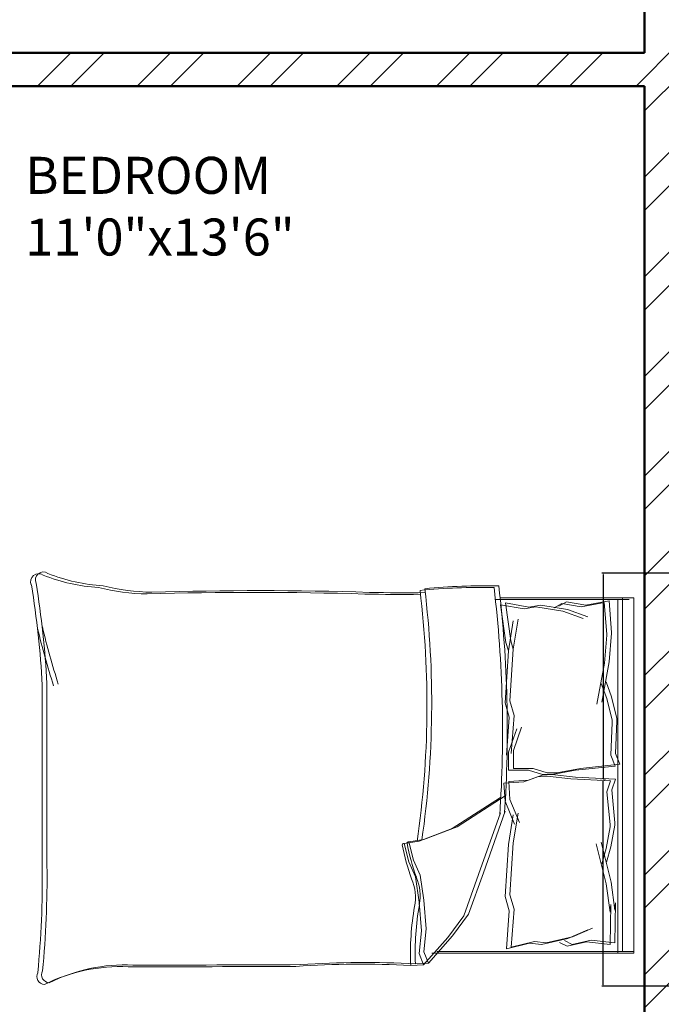
# Model space of a CAD drawing. Units: inches. Extents: x 963 to 2075, y 289 to 2657.
# Tile 12 of 98: x 1424 to 1511, y 1585 to 1718. Entities that reach past the tile are written whole.
import ezdxf

# ---------------------------------------------------------------- set-up
doc = ezdxf.new("R2010")
doc.units = ezdxf.units.IN
for name, color, linetype, lineweight in [('A-ANNO-DIMS', 2, 'Continuous', 18), ('A-AREA-IDEN', 7, 'Continuous', 18), ('A-FURN', 8, 'Continuous', 18), ('A-WALL', 7, 'Continuous', 50), ('A-WALL-PATT', 8, 'Continuous', 13)]:
    doc.layers.add(name, color=color, linetype=linetype, lineweight=lineweight)
doc.styles.get("Standard").update_dxf_attribs({"font": 'arial.ttf'})
doc.dimstyles.get("Standard").update_dxf_attribs({"dimtxt": 0.18, "dimasz": 0.18, "dimexe": 0.18, "dimexo": 0.0625, "dimgap": 0.09, "dimtad": 0, "dimtih": 1, "dimtoh": 1, "dimdec": 4, "dimzin": 0, "dimdsep": 46, "dimtxsty": 'Standard', "dimcen": 0.09, "dimadec": 0, "dimazin": 0, "dimtfac": 1, "dimtdec": 4, "dimtofl": 0, "dimtmove": 0, "dimatfit": 3, "dimfxl": 1, "dimtolj": 1, "dimtzin": 0, "dimarcsym": 0})

# ---------------------------------------------------------------- blocks, each defined once
blk = doc.blocks.new('BED-DOUBLE')
for p, q in [((1236.12, 2450.52), (1254.23, 2450.52)), ((1236.12, 2450.52), (1254.23, 2450.52)), ((1236.76, 2450.75), (1254.87, 2450.75)), ((1236.76, 2450.75), (1254.87, 2450.75)), ((1237.61, 2444.71), (1236.89, 2449.81)), ((1236.89, 2449.81), (1240.07, 2449.23)), ((1237.61, 2444.71), (1236.89, 2449.81)), ((1236.89, 2449.81), (1240.07, 2449.23)), ((1238.25, 2444.94), (1237.53, 2450.04)), ((1237.53, 2450.04), (1240.71, 2449.46)), ((1238.25, 2444.94), (1237.53, 2450.04)), ((1237.53, 2450.04), (1240.71, 2449.46)), ((1240.07, 2449.23), (1241.66, 2449.52)), ((1240.07, 2449.23), (1241.66, 2449.52)), ((1240.71, 2449.46), (1242.3, 2449.75)), ((1240.71, 2449.46), (1242.3, 2449.75)), ((1241.66, 2449.52), (1245.28, 2448.94)), ((1241.66, 2449.52), (1245.28, 2448.94)), ((1242.3, 2449.75), (1245.92, 2449.17)), ((1242.3, 2449.75), (1245.92, 2449.17)), ((1245.13, 2449.96), (1244.12, 2449.38)), ((1245.13, 2449.96), (1244.12, 2449.38)), ((1245.77, 2450.18), (1244.76, 2449.61)), ((1245.77, 2450.18), (1244.76, 2449.61)), ((1247.74, 2449.52), (1245.13, 2449.96)), ((1247.74, 2449.52), (1245.13, 2449.96)), ((1248.37, 2449.75), (1245.77, 2450.18)), ((1248.37, 2449.75), (1245.77, 2450.18)), ((1250.92, 2450.1), (1247.74, 2449.52)), ((1250.92, 2450.1), (1247.74, 2449.52)), ((1251.56, 2450.33), (1248.37, 2449.75)), ((1251.56, 2450.33), (1248.37, 2449.75)), ((1250.89, 2450.1), (1251.22, 2445.82)), ((1250.89, 2450.1), (1251.22, 2445.82)), ((1251.53, 2450.32), (1251.86, 2446.04)), ((1251.53, 2450.32), (1251.86, 2446.04)), ((1252.7, 2450.52), (1252.7, 2402.73)), ((1252.7, 2450.52), (1252.7, 2402.73)), ((1253.34, 2450.75), (1253.34, 2402.96)), ((1253.34, 2450.75), (1253.34, 2402.96)), ((1254.87, 2450.75), (1254.87, 2402.73)), ((1245.28, 2448.94), (1248.02, 2447.93)), ((1245.28, 2448.94), (1248.02, 2447.93)), ((1245.92, 2449.17), (1248.66, 2448.16)), ((1245.92, 2449.17), (1248.66, 2448.16)), ((1238.6, 2447.61), (1237.94, 2443.58)), ((1238.6, 2447.61), (1237.94, 2443.58)), ((1239.24, 2447.84), (1238.58, 2443.81)), ((1239.24, 2447.84), (1238.58, 2443.81)), ((1251.21, 2445.71), (1250.92, 2441.89)), ((1251.21, 2445.71), (1250.92, 2441.89)), ((1251.22, 2445.82), (1251.21, 2445.71)), ((1251.22, 2445.82), (1251.21, 2445.71)), ((1251.84, 2445.94), (1251.56, 2442.11)), ((1251.84, 2445.94), (1251.56, 2442.11)), ((1251.86, 2446.04), (1251.84, 2445.94)), ((1251.86, 2446.04), (1251.84, 2445.94)), ((1237.94, 2443.58), (1237.61, 2444.71)), ((1237.94, 2443.58), (1237.61, 2444.71)), ((1238.58, 2443.81), (1238.25, 2444.94)), ((1238.58, 2443.81), (1238.25, 2444.94)), ((1237.94, 2443.58), (1237.51, 2436.57)), ((1237.94, 2443.58), (1237.51, 2436.57)), ((1238.58, 2443.81), (1238.15, 2436.8)), ((1238.58, 2443.81), (1238.15, 2436.8)), ((1250.92, 2441.89), (1249.9, 2436.39)), ((1250.92, 2441.89), (1249.9, 2436.39)), ((1251.56, 2442.11), (1250.54, 2436.62)), ((1251.56, 2442.11), (1250.54, 2436.62)), ((1174.99, 2438.93), (1174.99, 2414.32)), ((1174.99, 2438.93), (1174.99, 2414.32)), ((1175.63, 2439.16), (1175.63, 2414.55)), ((1175.63, 2439.16), (1175.63, 2414.55)), ((1250.48, 2439.14), (1251.21, 2437.12)), ((1250.48, 2439.14), (1251.21, 2437.12)), ((1251.12, 2439.37), (1251.84, 2437.34)), ((1251.12, 2439.37), (1251.84, 2437.34)), ((1237.51, 2436.57), (1238.06, 2434.61)), ((1237.51, 2436.57), (1238.06, 2434.61)), ((1238.15, 2436.8), (1238.7, 2434.84)), ((1238.15, 2436.8), (1238.7, 2434.84)), ((1251.21, 2437.12), (1251.93, 2434.22)), ((1251.21, 2437.12), (1251.93, 2434.23)), ((1251.84, 2437.34), (1252.57, 2434.45)), ((1251.84, 2437.34), (1252.57, 2434.45)), ((1238.06, 2434.61), (1237.66, 2429.48)), ((1238.06, 2434.61), (1237.66, 2429.48)), ((1238.7, 2434.84), (1238.3, 2429.71)), ((1238.7, 2434.84), (1238.3, 2429.71)), ((1251.93, 2433.9), (1251.78, 2429.46)), ((1251.93, 2433.9), (1251.78, 2429.46)), ((1251.93, 2434.23), (1251.93, 2433.9)), ((1251.93, 2434.22), (1251.93, 2433.9)), ((1252.57, 2434.13), (1252.42, 2429.69)), ((1252.57, 2434.13), (1252.42, 2429.69)), ((1252.57, 2434.45), (1252.57, 2434.13)), ((1252.57, 2434.45), (1252.57, 2434.13)), ((1237.97, 2429.89), (1239.06, 2433.04)), ((1237.97, 2429.89), (1239.06, 2433.04)), ((1238.61, 2430.12), (1239.7, 2433.26)), ((1238.61, 2430.12), (1239.7, 2433.26)), ((1237.97, 2427.43), (1237.97, 2429.89)), ((1237.97, 2427.43), (1237.97, 2429.89)), ((1238.61, 2427.66), (1238.61, 2430.12)), ((1238.61, 2427.66), (1238.61, 2430.12)), ((1252.42, 2429.69), (1253, 2428.24)), ((1252.42, 2429.69), (1253, 2428.24)), ((1253, 2428.24), (1247.65, 2427.66)), ((1253, 2428.24), (1247.65, 2427.66)), ((1251.78, 2429.46), (1252.36, 2428.01)), ((1251.78, 2429.46), (1252.36, 2428.01)), ((1240.65, 2427.43), (1237.97, 2427.43)), ((1240.65, 2427.43), (1237.97, 2427.43)), ((1241.29, 2427.66), (1238.61, 2427.66)), ((1241.29, 2427.66), (1238.61, 2427.66)), ((1242.53, 2426.86), (1240.65, 2427.43)), ((1242.53, 2426.86), (1240.65, 2427.43)), ((1243.17, 2427.08), (1241.29, 2427.66)), ((1243.17, 2427.08), (1241.29, 2427.66)), ((1244.47, 2427.08), (1243.17, 2427.08)), ((1244.47, 2427.08), (1243.17, 2427.08)), ((1247.01, 2427.43), (1243.83, 2426.86)), ((1247.01, 2427.43), (1243.83, 2426.86)), ((1247.65, 2427.66), (1244.47, 2427.08)), ((1247.65, 2427.66), (1244.47, 2427.08)), ((1252.36, 2428.01), (1247.01, 2427.43)), ((1252.36, 2428.01), (1247.01, 2427.43)), ((1240.02, 2425.86), (1237.34, 2425.7)), ((1240.02, 2425.86), (1237.34, 2425.7)), ((1237.34, 2425.7), (1237.49, 2423.24)), ((1237.34, 2425.7), (1237.49, 2423.24)), ((1240.66, 2426.09), (1237.98, 2425.93)), ((1240.66, 2426.09), (1237.98, 2425.93)), ((1237.98, 2425.93), (1238.13, 2423.47)), ((1237.98, 2425.93), (1238.13, 2423.47)), ((1241.86, 2426.56), (1240.02, 2425.86)), ((1241.86, 2426.56), (1240.02, 2425.86)), ((1242.49, 2426.79), (1240.66, 2426.09)), ((1242.49, 2426.79), (1240.66, 2426.09)), ((1243.15, 2426.64), (1241.86, 2426.56)), ((1243.15, 2426.64), (1241.86, 2426.56)), ((1243.79, 2426.87), (1242.49, 2426.79)), ((1243.79, 2426.87), (1242.49, 2426.79)), ((1243.83, 2426.86), (1242.53, 2426.86)), ((1243.83, 2426.86), (1242.53, 2426.86)), ((1246.37, 2426.26), (1243.15, 2426.64)), ((1246.37, 2426.26), (1243.15, 2426.64)), ((1247, 2426.49), (1243.79, 2426.87)), ((1247, 2426.49), (1243.79, 2426.87)), ((1251.74, 2426.02), (1246.37, 2426.26)), ((1251.74, 2426.02), (1246.37, 2426.26)), ((1252.38, 2426.25), (1247, 2426.49)), ((1252.38, 2426.25), (1247, 2426.49)), ((1251.25, 2424.54), (1251.74, 2426.02)), ((1251.25, 2424.54), (1251.74, 2426.02)), ((1251.89, 2424.77), (1252.38, 2426.25)), ((1251.89, 2424.77), (1252.38, 2426.25)), ((1251.68, 2420.11), (1251.25, 2424.54)), ((1251.68, 2420.11), (1251.25, 2424.54)), ((1252.31, 2420.34), (1251.89, 2424.77)), ((1252.31, 2420.34), (1251.89, 2424.77)), ((1236.85, 2423.74), (1230.36, 2419.55)), ((1236.85, 2423.74), (1230.36, 2419.55)), ((1237.49, 2423.96), (1231, 2419.77)), ((1237.49, 2423.96), (1231, 2419.77)), ((1237.49, 2423.24), (1238.78, 2420.17)), ((1237.49, 2423.24), (1238.78, 2420.17)), ((1238.13, 2423.47), (1239.42, 2420.4)), ((1238.13, 2423.47), (1239.42, 2420.4)), ((1233.92, 2413.35), (1236.85, 2421.69)), ((1233.92, 2413.35), (1236.85, 2421.69)), ((1234.56, 2413.58), (1237.49, 2421.92)), ((1234.56, 2413.58), (1237.49, 2421.92)), ((1239.24, 2421.66), (1238.58, 2417.63)), ((1239.24, 2421.66), (1238.58, 2417.63)), ((1238.6, 2421.43), (1237.94, 2417.4)), ((1238.6, 2421.43), (1237.94, 2417.4)), ((1252.33, 2420.02), (1252.31, 2420.34)), ((1252.33, 2420.02), (1252.31, 2420.34)), ((1230.36, 2419.55), (1225.87, 2417.84)), ((1230.36, 2419.55), (1225.87, 2417.84)), ((1231, 2419.77), (1226.51, 2418.07)), ((1231, 2419.77), (1226.51, 2418.07)), ((1251.15, 2416.86), (1251.7, 2419.79)), ((1251.15, 2416.86), (1251.7, 2419.79)), ((1251.7, 2419.79), (1251.68, 2420.11)), ((1251.7, 2419.79), (1251.68, 2420.11)), ((1251.79, 2417.09), (1252.33, 2420.02)), ((1251.79, 2417.09), (1252.33, 2420.02)), ((1225.87, 2417.84), (1223.86, 2417.53)), ((1225.87, 2417.84), (1223.86, 2417.53)), ((1226.51, 2418.07), (1224.49, 2417.76)), ((1226.51, 2418.07), (1224.49, 2417.76)), ((1224.49, 2417.76), (1225.11, 2415.28)), ((1224.49, 2417.76), (1225.11, 2415.28)), ((1238.58, 2417.63), (1238.15, 2410.62)), ((1238.58, 2417.63), (1238.15, 2410.62)), ((1251.8, 2412.31), (1250.45, 2417.73)), ((1251.8, 2412.31), (1250.45, 2417.73)), ((1223.86, 2417.53), (1224.47, 2415.05)), ((1223.86, 2417.53), (1224.47, 2415.05)), ((1237.94, 2417.4), (1237.51, 2410.39)), ((1237.94, 2417.4), (1237.51, 2410.39)), ((1251.16, 2412.08), (1249.81, 2417.5)), ((1251.16, 2412.08), (1249.81, 2417.5)), ((1250.56, 2414.79), (1251.15, 2416.86)), ((1250.56, 2414.79), (1251.15, 2416.86)), ((1251.2, 2415.02), (1251.79, 2417.09)), ((1251.2, 2415.02), (1251.79, 2417.09)), ((1224.47, 2415.05), (1225.4, 2413.04)), ((1224.47, 2415.05), (1225.4, 2413.04)), ((1225.11, 2415.28), (1226.04, 2413.27)), ((1225.11, 2415.28), (1226.04, 2413.27)), ((1232.54, 2408), (1234.56, 2413.58)), ((1232.54, 2408), (1234.56, 2413.58)), ((1225.4, 2413.04), (1225.87, 2409.63)), ((1225.4, 2413.04), (1225.87, 2409.63)), ((1226.04, 2413.27), (1226.51, 2409.86)), ((1226.04, 2413.27), (1226.51, 2409.86)), ((1231.9, 2407.77), (1233.92, 2413.35)), ((1231.9, 2407.78), (1233.92, 2413.35)), ((1252.33, 2408.51), (1251.8, 2412.31)), ((1252.33, 2408.51), (1251.8, 2412.31)), ((1251.69, 2408.28), (1251.16, 2412.08)), ((1251.69, 2408.28), (1251.16, 2412.08)), ((1225.87, 2409.63), (1226.18, 2405.76)), ((1225.87, 2409.63), (1226.18, 2405.76)), ((1226.51, 2409.86), (1226.82, 2405.99)), ((1226.51, 2409.86), (1226.82, 2405.99)), ((1237.51, 2410.39), (1238.06, 2408.43)), ((1237.51, 2410.39), (1238.06, 2408.43)), ((1238.15, 2410.62), (1238.7, 2408.66)), ((1238.15, 2410.62), (1238.7, 2408.66)), ((1238.06, 2408.43), (1237.66, 2403.3)), ((1238.06, 2408.43), (1237.66, 2403.3)), ((1238.7, 2408.66), (1238.3, 2403.52)), ((1238.7, 2408.66), (1238.3, 2403.52)), ((1251.68, 2403.88), (1251.77, 2409.29)), ((1251.68, 2403.88), (1251.77, 2409.28)), ((1251.77, 2409.29), (1251.69, 2408.28)), ((1251.77, 2409.28), (1251.69, 2408.28)), ((1252.31, 2404.11), (1252.41, 2409.51)), ((1252.31, 2404.11), (1252.41, 2409.51)), ((1252.41, 2409.51), (1252.33, 2408.51)), ((1252.41, 2409.51), (1252.33, 2408.51)), ((1229.74, 2404.83), (1231.9, 2407.78)), ((1229.74, 2404.83), (1231.9, 2407.77)), ((1230.38, 2405.06), (1232.54, 2408)), ((1230.38, 2405.06), (1232.54, 2408)), ((1226.18, 2405.76), (1225.87, 2402.66)), ((1226.18, 2405.76), (1225.87, 2402.66)), ((1226.82, 2405.99), (1226.51, 2402.89)), ((1226.82, 2405.99), (1226.51, 2402.89)), ((1245.98, 2404.69), (1248.65, 2405.87)), ((1245.98, 2404.69), (1248.65, 2405.87)), ((1246.61, 2404.91), (1249.29, 2406.1)), ((1246.61, 2404.91), (1249.29, 2406.09)), ((1226.49, 2401.13), (1229.74, 2404.83)), ((1226.49, 2401.13), (1229.74, 2404.83)), ((1227.13, 2401.36), (1230.38, 2405.06)), ((1227.13, 2401.36), (1230.38, 2405.06)), ((1238.3, 2403.52), (1241.44, 2404.3)), ((1238.3, 2403.52), (1241.44, 2404.3)), ((1241.44, 2404.3), (1243.04, 2404.11)), ((1241.44, 2404.3), (1243.04, 2404.11)), ((1242.4, 2403.88), (1245.98, 2404.69)), ((1242.4, 2403.88), (1245.98, 2404.69)), ((1243.04, 2404.11), (1246.61, 2404.91)), ((1243.04, 2404.11), (1246.61, 2404.91)), ((1246.53, 2403.89), (1245.49, 2404.41)), ((1246.53, 2403.89), (1245.49, 2404.41)), ((1248.46, 2404.26), (1245.89, 2403.67)), ((1248.46, 2404.26), (1245.89, 2403.67)), ((1249.1, 2404.49), (1246.53, 2403.89)), ((1249.1, 2404.49), (1246.53, 2403.89)), ((1251.68, 2403.88), (1248.46, 2404.26)), ((1251.68, 2403.88), (1248.46, 2404.26)), ((1252.31, 2404.11), (1249.1, 2404.49)), ((1252.31, 2404.11), (1249.1, 2404.49)), ((1254.87, 2402.96), (1228.26, 2402.96)), ((1254.87, 2402.96), (1228.26, 2402.96)), ((1237.66, 2403.3), (1240.8, 2404.07)), ((1237.66, 2403.3), (1240.8, 2404.07)), ((1240.8, 2404.07), (1242.4, 2403.88)), ((1240.8, 2404.07), (1242.4, 2403.88)), ((1245.89, 2403.67), (1244.85, 2404.18)), ((1245.89, 2403.67), (1244.85, 2404.18)), ((1225.87, 2402.66), (1226.49, 2401.13)), ((1225.87, 2402.66), (1226.49, 2401.13)), ((1226.51, 2402.89), (1227.13, 2401.36)), ((1226.51, 2402.89), (1227.13, 2401.36)), ((1254.23, 2402.73), (1227.62, 2402.73)), ((1254.23, 2402.73), (1227.62, 2402.73)), ((1254.87, 2402.73), (1254.23, 2402.73)), ((1224.74, 2401.05), (1226.49, 2401.13, 3.87)), ((1224.74, 2401.05), (1226.49, 2401.13, 3.87)), ((1225.38, 2401.28), (1227.13, 2401.36, 3.87)), ((1225.38, 2401.28), (1227.13, 2401.36, 3.87))]:
    blk.add_line(p, q)
for centre, radius, start, end in [((1174.51, 2452.91), 1.09, 56.1736, 203.4781), ((1174.51, 2452.91), 1.09, 56.1736, 203.4781), ((1175.15, 2453.14), 1.09, 56.1736, 203.4781), ((1175.15, 2453.14), 1.09, 56.1736, 203.4781), ((1183.96, 2475.65), 23.56, 247.9751, 266.652), ((1183.96, 2475.65), 23.56, 247.9751, 266.652), ((1184.6, 2475.88), 23.56, 247.9751, 266.652), ((1184.6, 2475.88), 23.56, 247.9751, 266.652), ((1053.4, 2432.57), 121.76, 2.9958, 9.4091), ((1053.4, 2432.57), 121.76, 2.9958, 9.4091), ((1054.03, 2432.8), 121.76, 2.9958, 9.4091), ((1054.03, 2432.8), 121.76, 2.9958, 9.4091), ((1190.36, 2481.12), 29.63, 256.0648, 268.9113), ((1190.36, 2481.12), 29.63, 256.0648, 268.9113), ((1234.78, 2369.06), 83.31, 88.7218, 95.604), ((1234.78, 2369.06), 83.31, 88.7218, 95.604), ((1072.82, 2432.86), 164.97, 356.0865, 6.7821), ((1072.82, 2432.86), 164.97, 356.0865, 6.7821), ((1189.72, 2480.89), 29.63, 256.0648, 268.9113), ((1189.72, 2480.89), 29.63, 256.0648, 268.9113), ((1203.62, 1969.17), 482.31, 88.2277, 91.7185), ((1203.62, 1969.17), 482.31, 88.2277, 91.7185), ((1204.26, 1969.4), 482.31, 88.2277, 91.7185), ((1204.26, 1969.4), 482.31, 88.2277, 91.7185), ((1223.06, 2621.3), 170.11, 268.4762, 271.0082), ((1223.06, 2621.3), 170.11, 268.4762, 271.0082), ((1223.7, 2621.53), 170.11, 268.4762, 271.0082), ((1223.7, 2621.53), 170.11, 268.4762, 271.0082), ((1097.92, 2436.24), 129.02, 351.7845, 6.9006), ((1097.92, 2436.24), 129.02, 351.7845, 6.9006), ((1234.14, 2368.83), 83.31, 88.7218, 95.604), ((1234.14, 2368.83), 83.31, 88.7218, 95.604), ((1098.56, 2436.47), 129.02, 351.7845, 6.9006), ((1098.56, 2436.47), 129.02, 351.7845, 6.9006), ((1072.18, 2432.64), 164.97, 356.0865, 6.7821), ((1072.18, 2432.64), 164.97, 356.0865, 6.7821), ((1277.94, 2471.22), 106.46, 193.3832, 197.7053), ((1277.94, 2471.22), 106.46, 193.3832, 197.7053), ((1278.58, 2471.44), 106.46, 193.3832, 197.7053), ((1278.58, 2471.44), 106.46, 193.3832, 197.7053), ((1224.43, 2417.59), 0.185, 70.2464, 181.1377), ((1224.43, 2417.59), 0.185, 70.2464, 181.1377), ((1253.39, 2423.07), 29.65, 190.6617, 199.8806), ((1253.39, 2423.07), 29.65, 190.6617, 199.8806), ((1223.79, 2417.36), 0.185, 70.2464, 181.1377), ((1223.79, 2417.36), 0.185, 70.2464, 181.1377), ((1252.75, 2422.84), 29.65, 190.6617, 199.8806), ((1252.75, 2422.84), 29.65, 190.6617, 199.8806), ((1041.96, 2412.84), 133.04, 354.4998, 0.6351), ((1041.96, 2412.84), 133.04, 354.4998, 0.6351), ((1042.6, 2413.07), 133.04, 354.4998, 0.6351), ((1042.6, 2413.07), 133.04, 354.4998, 0.6351), ((1219.17, 2410.25), 6.22, 348.6608, 23.7384), ((1219.17, 2410.25), 6.22, 348.6608, 23.7384), ((1219.81, 2410.48), 6.22, 348.6608, 23.7384), ((1219.81, 2410.48), 6.22, 348.6608, 23.7384), ((1260.89, 2402.67), 36.18, 169.8763, 182.5657), ((1260.89, 2402.67), 36.18, 169.8763, 182.5657), ((1261.53, 2402.9), 36.18, 169.8763, 182.5657), ((1261.53, 2402.9), 36.18, 169.8763, 182.5657), ((1176, 2399.81), 1.1, 152.6588, 266.02), ((1176, 2399.81), 1.1, 152.6588, 266.02), ((1185.57, 2377.84), 23.07, 87.4714, 116.4681), ((1185.57, 2377.84), 23.07, 87.4714, 116.4681), ((1186.21, 2378.07), 23.07, 87.4714, 116.4681), ((1186.21, 2378.07), 23.07, 87.4714, 116.4681), ((1186.41, 6962.74), 4561.86, 270.00217, 270.28689), ((1186.41, 6962.74), 4561.86, 270.00217, 270.28689), ((1187.05, 6962.97), 4561.86, 270.00217, 270.28689), ((1187.05, 6962.97), 4561.86, 270.00217, 270.28689), ((1217.92, 2271.73), 129.5, 86.9791, 93.8365), ((1217.92, 2271.73), 129.5, 86.9791, 93.8365), ((1218.56, 2271.96), 129.5, 86.9791, 93.8365), ((1218.56, 2271.96), 129.5, 86.9791, 93.8365), ((1175.36, 2399.58), 1.1, 152.6588, 266.02), ((1175.36, 2399.58), 1.1, 152.6588, 266.02)]:
    blk.add_arc(centre, radius, start, end)
blk = doc.blocks.new('*D15')
at = {"layer": 'A-ANNO-DIMS', "color": 0, "lineweight": -2, "transparency": 16777216}
for p, q in [((1515, 1643.51), (1502.65, 1643.51)), ((1502.83, 1643.33), (1502.83, 1615.78)), ((1502.83, 1587.86), (1502.83, 1615.41)), ((1515, 1587.68), (1502.65, 1587.68))]:
    blk.add_line(p, q, dxfattribs=at)
at = {"layer": 'A-ANNO-DIMS', "color": 0, "transparency": 16777216}
for points in [[(1502.8, 1643.33), (1502.86, 1643.33), (1502.83, 1643.51)], [(1502.8, 1587.86), (1502.86, 1587.86), (1502.83, 1587.68)]]:
    blk.add_solid(points, dxfattribs=at)
at = {"layer": 'Defpoints', "color": 0, "transparency": 16777216}
for p in [(1515.07, 1643.51), (1502.83, 1587.68), (1515.07, 1587.68)]:
    blk.add_point(p, dxfattribs=at)
at = {"layer": 'A-ANNO-DIMS', "color": 0, "transparency": 16777216, "insert": (1502.83, 1615.59), "char_height": 0.18, "attachment_point": 5}
blk.add_mtext('\\A1;56 TYP.', dxfattribs=at)

msp = doc.modelspace()

# ---------------------------------------------------------------- hatches: boundary and pattern name
at = {"layer": 'A-WALL-PATT'}
h = msp.add_hatch(dxfattribs=at)
h.set_pattern_fill('ANSI32', color=256)
h.paths.add_polyline_path([(1296.92, 2558.32), (1203.92, 2558.32), (1203.92, 2493.82), (1191.53, 2493.82), (1191.53, 2489.32), (1211.06, 2489.32), (1211.06, 2492.02), (1211.06, 2493.82), (1208.42, 2493.82), (1208.42, 2553.82), (1292.42, 2553.82), (1292.42, 2538.86), (1296.92, 2538.86)])
h.paths.add_polyline_path([(1442.42, 2558.32), (1349.42, 2558.32), (1349.42, 2538.94), (1353.92, 2538.94), (1353.92, 2553.82), (1437.92, 2553.82), (1437.92, 2493.82), (1434.54, 2493.82), (1434.54, 2489.32), (1448.31, 2489.32), (1448.31, 2491.57), (1448.31, 2493.82), (1442.42, 2493.82)])
h.paths.add_polyline_path([(1415.55, 2491.57), (1415.55, 2493.82), (1340.94, 2493.82), (1340.94, 2489.32), (1371.92, 2489.32), (1371.92, 2378.32), (1367.6, 2378.32), (1367.6, 2373.82), (1371.92, 2373.82), (1371.92, 2355.19), (1376.42, 2355.19), (1376.42, 2489.32), (1415.55, 2489.32)])
h.paths.add_polyline_path([(1304.94, 2491.57), (1304.94, 2493.82), (1296.92, 2493.82), (1296.92, 2514.86), (1292.42, 2514.86), (1292.42, 2493.82), (1232.81, 2493.82), (1232.81, 2489.32), (1256.42, 2489.32), (1256.42, 2327.32), (1253.71, 2327.32), (1253.71, 2322.82), (1328.42, 2322.82), (1328.42, 2331.15), (1323.92, 2331.15), (1323.92, 2327.32), (1260.92, 2327.32), (1260.92, 2373.82), (1323.92, 2373.82), (1323.92, 2357.81), (1328.42, 2357.81), (1328.42, 2373.82), (1346.01, 2373.82), (1346.01, 2376.07), (1346.01, 2378.32), (1260.92, 2378.32), (1260.92, 2489.32), (1304.94, 2489.32)])
h.paths.add_polyline_path([(1226.65, 2327.32), (1124.42, 2327.32), (1124.42, 2347.45), (1119.92, 2347.45), (1119.92, 2322.82), (1163.42, 2322.82), (1163.42, 2305.43), (1165.67, 2305.43), (1167.92, 2305.43), (1167.92, 2322.82), (1226.65, 2322.82), (1226.65, 2325.07)])
h.paths.add_polyline_path([(1095.92, 2489.32), (1124.42, 2489.32), (1131.53, 2489.32), (1131.53, 2491.57), (1131.53, 2493.82), (1119.92, 2493.82), (1091.42, 2493.82), (1091.42, 2417.32), (1095.92, 2417.32), (1119.92, 2417.32), (1119.92, 2407.45), (1124.42, 2407.45), (1124.42, 2421.82), (1095.92, 2421.82)])
h.paths.add_polyline_path([(1512.92, 2558.32), (1508.42, 2558.32), (1508.42, 2493.82), (1503.4, 2493.82), (1503.4, 2489.32), (1508.42, 2489.32), (1508.42, 2327.32), (1376.42, 2327.32), (1376.42, 2330.27), (1371.92, 2330.27), (1371.92, 2298.74), (1376.42, 2298.74), (1376.42, 2322.82), (1508.42, 2322.82), (1508.42, 2165.32), (1504.26, 2165.32), (1504.26, 2160.82), (1508.42, 2160.82), (1508.42, 2108.32), (1512.92, 2108.32), (1512.92, 2160.82), (1516.18, 2160.82), (1516.18, 2163.07), (1516.18, 2165.32), (1512.92, 2165.32), (1512.92, 2322.82), (1644.92, 2322.82), (1644.92, 2298.74), (1649.42, 2298.74), (1649.42, 2322.82), (1649.42, 2330.94), (1647.17, 2330.94), (1644.92, 2330.94), (1644.92, 2327.32), (1512.92, 2327.32), (1512.92, 2489.32), (1516.76, 2489.32), (1516.76, 2491.57), (1516.76, 2493.82), (1512.92, 2493.82)])
h.paths.add_polyline_path([(1671.92, 2558.32), (1578.92, 2558.32), (1578.92, 2493.82), (1573.53, 2493.82), (1573.53, 2489.32), (1586.54, 2489.32), (1586.54, 2491.57), (1586.54, 2493.82), (1583.42, 2493.82), (1583.42, 2553.82), (1667.42, 2553.82), (1667.42, 2541.11), (1671.92, 2541.11)])
h.paths.add_polyline_path([(1681.26, 2493.82), (1671.92, 2493.82), (1671.92, 2517.11), (1667.42, 2517.11), (1667.42, 2493.82), (1610.22, 2493.82), (1610.22, 2489.32), (1644.92, 2489.32), (1644.92, 2357.87), (1649.42, 2357.87), (1649.42, 2373.82), (1652.2, 2373.82), (1652.2, 2375.83), (1652.2, 2378.32), (1649.42, 2378.32), (1649.42, 2489.32), (1681.26, 2489.32), (1681.26, 2491.57)])
h.paths.add_polyline_path([(1821.92, 2558.32), (1728.92, 2558.32), (1728.92, 2541), (1733.42, 2541), (1733.42, 2553.82), (1817.42, 2553.82), (1817.42, 2493.82), (1813.51, 2493.82), (1813.51, 2489.32), (1830.08, 2489.32), (1830.08, 2491.57), (1830.08, 2493.82), (1821.92, 2493.82)])
h.paths.add_polyline_path([(1794.24, 2493.82), (1717.26, 2493.82), (1717.26, 2489.32), (1760.42, 2489.32), (1760.42, 2378.32), (1674.4, 2378.32), (1674.4, 2373.82), (1692.92, 2373.82), (1692.92, 2356.95), (1697.42, 2356.95), (1697.42, 2373.82), (1760.42, 2373.82), (1760.42, 2327.32), (1697.42, 2327.32), (1697.42, 2333.34), (1692.92, 2333.34), (1692.92, 2322.82), (1768.04, 2322.82), (1768.04, 2325.07), (1768.04, 2327.32), (1764.92, 2327.32), (1764.92, 2489.32), (1794.24, 2489.32)])
h.paths.add_polyline_path([(1733.42, 2517), (1728.92, 2517), (1728.92, 2493.82), (1733.42, 2493.82)], flags=17)
h.paths.add_polyline_path([(1929.92, 2493.82), (1890.08, 2493.82), (1890.08, 2489.32), (1896.92, 2489.32), (1925.42, 2489.32), (1925.42, 2421.82), (1896.92, 2421.82), (1896.92, 2408.32), (1901.42, 2408.32), (1901.42, 2417.32), (1925.42, 2417.32), (1929.92, 2417.32)])
h.paths.add_polyline_path([(1901.42, 2348.32), (1896.92, 2348.32), (1896.92, 2327.32), (1800.42, 2327.32), (1800.42, 2322.82), (1853.42, 2322.82), (1853.42, 2309.45), (1857.92, 2309.45), (1857.92, 2322.82), (1901.42, 2322.82)])
h.paths.add_polyline_path([(1857.92, 2249.45), (1853.42, 2249.45), (1853.42, 2214.82), (1686.31, 2214.82), (1686.31, 2210.32), (1853.42, 2210.32), (1853.42, 2202.13), (1857.92, 2202.13), (1857.92, 2210.32)])
h.paths.add_polyline_path([(1857.92, 2142.13), (1853.42, 2142.13), (1853.42, 2115.42), (1841.42, 2115.42), (1841.42, 2088.53), (1841.42, 2046.95), (1845.92, 2046.95), (1845.92, 2110.92), (1905.92, 2110.92), (1905.92, 2092.52), (1910.42, 2092.52), (1910.42, 2115.42), (1857.92, 2115.42)])
h.paths.add_polyline_path([(1532.44, 1482.34), (1573.46, 1482.34), (1573.46, 1501), (1532.44, 1501)], flags=9)
h.paths.add_polyline_path([(1438.66, 1486.3), (1479.68, 1486.3), (1479.68, 1504.96), (1438.66, 1504.96)], flags=9)
h.paths.add_polyline_path([(1411.22, 1365.31), (1659.14, 1365.31), (1659.14, 1402.4), (1411.22, 1402.4)], flags=9)
h.paths.add_polyline_path([(1185.67, 2296.3), (1248.16, 2296.3), (1248.16, 2314.95), (1185.67, 2314.95)], flags=9)
h.paths.add_polyline_path([(1177.31, 2187.35), (1216.15, 2187.35), (1216.15, 2206.01), (1177.31, 2206.01)], flags=9)
h.paths.add_polyline_path([(1295.1, 1602.08), (1328.26, 1602.08), (1328.26, 1620.74), (1295.1, 1620.74)], flags=9)
h.paths.add_polyline_path([(1525.13, 2005.99), (1558.39, 2005.99), (1558.39, 2024.65), (1525.13, 2024.65)], flags=9)
h.paths.add_polyline_path([(1459.61, 1977.13), (1472.19, 1977.13), (1472.19, 1987.43), (1459.61, 1987.43)], flags=9)
h.paths.add_polyline_path([(1467.81, 2053.68), (1480.02, 2053.68), (1480.02, 2063.98), (1467.81, 2063.98)], flags=9)
h.paths.add_polyline_path([(1555.18, 2119.02), (1584.56, 2119.02), (1584.56, 2137.68), (1555.18, 2137.68)], flags=25)
h.paths.add_polyline_path([(1405.39, 2115.29), (1444.48, 2115.29), (1444.48, 2133.95), (1405.39, 2133.95)], flags=25)
h.paths.add_polyline_path([(1698.48, 2004.26), (1727.69, 2004.26), (1727.69, 2022.92), (1698.48, 2022.92)], flags=9)
h.paths.add_polyline_path([(1612.16, 1972.86), (1629.02, 1972.86), (1629.02, 1983.16), (1612.16, 1983.16)], flags=9)
h.paths.add_polyline_path([(1608.29, 2060.04), (1625.15, 2060.04), (1625.15, 2070.34), (1608.29, 2070.34)], flags=9)
h.paths.add_polyline_path([(1527.95, 1684.4), (1566.79, 1684.4), (1566.79, 1703.06), (1527.95, 1703.06)], flags=9)
h.paths.add_polyline_path([(1422.79, 1683.59), (1461.63, 1683.59), (1461.63, 1702.25), (1422.79, 1702.25)], flags=9)
h.paths.add_polyline_path([(1531.26, 1732.46), (1574.01, 1732.46), (1574.01, 1751.12), (1531.26, 1751.12)], flags=9)
h.paths.add_polyline_path([(1402.87, 1732.85), (1439.8, 1732.85), (1439.8, 1751.5), (1402.87, 1751.5)], flags=9)
h.paths.add_polyline_path([(1243.12, 1923.13), (1281.96, 1923.13), (1281.96, 1941.79), (1243.12, 1941.79)], flags=9)
h.paths.add_polyline_path([(1181.75, 1792.27), (1244.24, 1792.27), (1244.24, 1810.93), (1181.75, 1810.93)], flags=9)
h.paths.add_polyline_path([(1265.82, 1670.3), (1316.07, 1670.3), (1316.07, 1688.96), (1265.82, 1688.96)], flags=9)
h.paths.add_polyline_path([(1140.26, 1676.05), (1179.1, 1676.05), (1179.1, 1694.71), (1140.26, 1694.71)], flags=9)
h.paths.add_polyline_path([(1107.49, 1490.89), (1143.37, 1490.89), (1143.37, 1509.55), (1107.49, 1509.55)], flags=9)
h.paths.add_polyline_path([(1217.58, 1483.9), (1246.74, 1483.9), (1246.74, 1502.56), (1217.58, 1502.56)], flags=9)
h.paths.add_polyline_path([(1389.21, 1486.92), (1418.37, 1486.92), (1418.37, 1505.58), (1389.21, 1505.58)], flags=9)
h.paths.add_polyline_path([(1672.21, 1602.08), (1705.37, 1602.08), (1705.37, 1620.74), (1672.21, 1620.74)], flags=9)
h.paths.add_polyline_path([(1752.08, 1522.64), (1781.24, 1522.64), (1781.24, 1541.3), (1752.08, 1541.3)], flags=9)
h.paths.add_polyline_path([(1848.27, 1491.26), (1884.16, 1491.26), (1884.16, 1509.92), (1848.27, 1509.92)], flags=9)
h.paths.add_polyline_path([(1822.47, 1685.62), (1861.31, 1685.62), (1861.31, 1704.28), (1822.47, 1704.28)], flags=9)
h.paths.add_polyline_path([(1713.19, 1672.23), (1763.44, 1672.23), (1763.44, 1690.89), (1713.19, 1690.89)], flags=9)
h.paths.add_polyline_path([(1736.62, 1790.58), (1799.11, 1790.58), (1799.11, 1809.24), (1736.62, 1809.24)], flags=9)
h.paths.add_polyline_path([(1691.49, 1916.36), (1730.33, 1916.36), (1730.33, 1935.01), (1691.49, 1935.01)], flags=9)
h.paths.add_polyline_path([(1764.87, 1973.92), (1794.31, 1973.92), (1794.31, 1992.58), (1764.87, 1992.58)], flags=9)
h.paths.add_polyline_path([(1767.85, 2034.02), (1797.29, 2034.02), (1797.29, 2052.67), (1767.85, 2052.67)], flags=9)
h.paths.add_polyline_path([(1851.59, 2060.33), (1880.75, 2060.33), (1880.75, 2078.99), (1851.59, 2078.99)], flags=25)
h.paths.add_polyline_path([(1688.49, 2086.87), (1727.33, 2086.87), (1727.33, 2105.53), (1688.49, 2105.53)], flags=9)
h.paths.add_polyline_path([(1537.74, 2293.58), (1580.49, 2293.58), (1580.49, 2312.24), (1537.74, 2312.24)], flags=25)
h.paths.add_polyline_path([(1425.59, 2296.11), (1468.34, 2296.11), (1468.34, 2314.77), (1425.59, 2314.77)], flags=25)
h.paths.add_polyline_path([(1278.52, 2004.18), (1307.72, 2004.18), (1307.72, 2022.84), (1278.52, 2022.84)], flags=9)
h.paths.add_polyline_path([(1193.28, 1973.63), (1222.72, 1973.63), (1222.72, 1992.29), (1193.28, 1992.29)], flags=9)
h.paths.add_polyline_path([(1192.41, 2040.58), (1221.84, 2040.58), (1221.84, 2059.23), (1192.41, 2059.23)], flags=9)
h.paths.add_polyline_path([(1130.6, 1951.39), (1159.76, 1951.39), (1159.76, 1970.05), (1130.6, 1970.05)], flags=9)
h.paths.add_polyline_path([(1132.83, 2052.49), (1161.98, 2052.49), (1161.98, 2071.15), (1132.83, 2071.15)], flags=9)
h.paths.add_polyline_path([(1265.13, 2334.62), (1315.38, 2334.62), (1315.38, 2353.28), (1265.13, 2353.28)], flags=25)
h.paths.add_polyline_path([(1136.74, 2330.79), (1175.58, 2330.79), (1175.58, 2349.44), (1136.74, 2349.44)], flags=9)
h.paths.add_polyline_path([(1287.42, 2417.2), (1320.58, 2417.2), (1320.58, 2435.86), (1287.42, 2435.86)], flags=25)
h.paths.add_polyline_path([(1430.99, 2329.16), (1469.83, 2329.16), (1469.83, 2347.82), (1430.99, 2347.82)], flags=25)
h.paths.add_polyline_path([(1525.42, 2329.21), (1564.26, 2329.21), (1564.26, 2347.87), (1525.42, 2347.87)], flags=25)
h.paths.add_polyline_path([(1684.52, 2382.8), (1717.68, 2382.8), (1717.68, 2401.46), (1684.52, 2401.46)], flags=25)
h.paths.add_polyline_path([(1704.81, 2340.29), (1755.05, 2340.29), (1755.05, 2358.95), (1704.81, 2358.95)], flags=25)
h.paths.add_polyline_path([(1694.11, 2287.76), (1756.6, 2287.76), (1756.6, 2306.41), (1694.11, 2306.41)], flags=9)
h.paths.add_polyline_path([(1815.78, 2329.86), (1854.62, 2329.86), (1854.62, 2348.52), (1815.78, 2348.52)], flags=9)
h.paths.add_polyline_path([(1842.87, 2514.26), (1878.76, 2514.26), (1878.76, 2532.91), (1842.87, 2532.91)], flags=9)
h.paths.add_polyline_path([(1769.51, 2531.45), (1798.67, 2531.45), (1798.67, 2550.1), (1769.51, 2550.1)], flags=25)
h.paths.add_polyline_path([(1594.77, 2518.47), (1623.93, 2518.47), (1623.93, 2537.13), (1594.77, 2537.13)], flags=25)
h.paths.add_polyline_path([(1520.72, 2516.18), (1556.61, 2516.18), (1556.61, 2534.84), (1520.72, 2534.84)], flags=25)
h.paths.add_polyline_path([(1464.46, 2516.69), (1500.34, 2516.69), (1500.34, 2535.35), (1464.46, 2535.35)], flags=25)
h.paths.add_polyline_path([(1365.7, 2528.97), (1394.85, 2528.97), (1394.85, 2547.63), (1365.7, 2547.63)], flags=25)
h.paths.add_polyline_path([(1222.84, 2516.23), (1252, 2516.23), (1252, 2534.89), (1222.84, 2534.89)], flags=25)
h.paths.add_polyline_path([(1104.55, 2509.6), (1140.43, 2509.6), (1140.43, 2528.26), (1104.55, 2528.26)], flags=9)
h = msp.add_hatch(dxfattribs=at)
h.set_pattern_fill('ANSI32', color=256)
h.paths.add_polyline_path([(1335.97, 2212.57), (1335.97, 2214.82), (1167.92, 2214.82), (1167.92, 2245.43), (1163.42, 2245.43), (1163.42, 2210.32), (1163.42, 2194.81), (1167.92, 2194.81), (1167.92, 2210.32), (1335.97, 2210.32)])
h.paths.add_polyline_path([(1532.44, 1482.34), (1573.46, 1482.34), (1573.46, 1501), (1532.44, 1501)], flags=9)
h.paths.add_polyline_path([(1438.66, 1486.3), (1479.68, 1486.3), (1479.68, 1504.96), (1438.66, 1504.96)], flags=9)
h.paths.add_polyline_path([(1411.22, 1365.31), (1659.14, 1365.31), (1659.14, 1402.4), (1411.22, 1402.4)], flags=9)
h.paths.add_polyline_path([(1185.67, 2296.3), (1248.16, 2296.3), (1248.16, 2314.95), (1185.67, 2314.95)], flags=9)
h.paths.add_polyline_path([(1177.31, 2187.35), (1216.15, 2187.35), (1216.15, 2206.01), (1177.31, 2206.01)], flags=9)
h.paths.add_polyline_path([(1295.1, 1602.08), (1328.26, 1602.08), (1328.26, 1620.74), (1295.1, 1620.74)], flags=9)
h.paths.add_polyline_path([(1525.13, 2005.99), (1558.39, 2005.99), (1558.39, 2024.65), (1525.13, 2024.65)], flags=9)
h.paths.add_polyline_path([(1459.61, 1977.13), (1472.19, 1977.13), (1472.19, 1987.43), (1459.61, 1987.43)], flags=9)
h.paths.add_polyline_path([(1467.81, 2053.68), (1480.02, 2053.68), (1480.02, 2063.98), (1467.81, 2063.98)], flags=9)
h.paths.add_polyline_path([(1555.18, 2119.02), (1584.56, 2119.02), (1584.56, 2137.68), (1555.18, 2137.68)], flags=9)
h.paths.add_polyline_path([(1405.39, 2115.29), (1444.48, 2115.29), (1444.48, 2133.95), (1405.39, 2133.95)], flags=9)
h.paths.add_polyline_path([(1698.48, 2004.26), (1727.69, 2004.26), (1727.69, 2022.92), (1698.48, 2022.92)], flags=9)
h.paths.add_polyline_path([(1612.16, 1972.86), (1629.02, 1972.86), (1629.02, 1983.16), (1612.16, 1983.16)], flags=9)
h.paths.add_polyline_path([(1608.29, 2060.04), (1625.15, 2060.04), (1625.15, 2070.34), (1608.29, 2070.34)], flags=9)
h.paths.add_polyline_path([(1527.95, 1684.4), (1566.79, 1684.4), (1566.79, 1703.06), (1527.95, 1703.06)], flags=9)
h.paths.add_polyline_path([(1422.79, 1683.59), (1461.63, 1683.59), (1461.63, 1702.25), (1422.79, 1702.25)], flags=9)
h.paths.add_polyline_path([(1531.26, 1732.46), (1574.01, 1732.46), (1574.01, 1751.12), (1531.26, 1751.12)], flags=9)
h.paths.add_polyline_path([(1402.87, 1732.85), (1439.8, 1732.85), (1439.8, 1751.5), (1402.87, 1751.5)], flags=9)
h.paths.add_polyline_path([(1243.12, 1923.13), (1281.96, 1923.13), (1281.96, 1941.79), (1243.12, 1941.79)], flags=9)
h.paths.add_polyline_path([(1181.75, 1792.27), (1244.24, 1792.27), (1244.24, 1810.93), (1181.75, 1810.93)], flags=9)
h.paths.add_polyline_path([(1265.82, 1670.3), (1316.07, 1670.3), (1316.07, 1688.96), (1265.82, 1688.96)], flags=9)
h.paths.add_polyline_path([(1140.26, 1676.05), (1179.1, 1676.05), (1179.1, 1694.71), (1140.26, 1694.71)], flags=9)
h.paths.add_polyline_path([(1107.49, 1490.89), (1143.37, 1490.89), (1143.37, 1509.55), (1107.49, 1509.55)], flags=9)
h.paths.add_polyline_path([(1217.58, 1483.9), (1246.74, 1483.9), (1246.74, 1502.56), (1217.58, 1502.56)], flags=9)
h.paths.add_polyline_path([(1389.21, 1486.92), (1418.37, 1486.92), (1418.37, 1505.58), (1389.21, 1505.58)], flags=9)
h.paths.add_polyline_path([(1672.21, 1602.08), (1705.37, 1602.08), (1705.37, 1620.74), (1672.21, 1620.74)], flags=9)
h.paths.add_polyline_path([(1752.08, 1522.64), (1781.24, 1522.64), (1781.24, 1541.3), (1752.08, 1541.3)], flags=9)
h.paths.add_polyline_path([(1848.27, 1491.26), (1884.16, 1491.26), (1884.16, 1509.92), (1848.27, 1509.92)], flags=9)
h.paths.add_polyline_path([(1822.47, 1685.62), (1861.31, 1685.62), (1861.31, 1704.28), (1822.47, 1704.28)], flags=9)
h.paths.add_polyline_path([(1713.19, 1672.23), (1763.44, 1672.23), (1763.44, 1690.89), (1713.19, 1690.89)], flags=9)
h.paths.add_polyline_path([(1736.62, 1790.58), (1799.11, 1790.58), (1799.11, 1809.24), (1736.62, 1809.24)], flags=9)
h.paths.add_polyline_path([(1691.49, 1916.36), (1730.33, 1916.36), (1730.33, 1935.01), (1691.49, 1935.01)], flags=9)
h.paths.add_polyline_path([(1764.87, 1973.92), (1794.31, 1973.92), (1794.31, 1992.58), (1764.87, 1992.58)], flags=9)
h.paths.add_polyline_path([(1767.85, 2034.02), (1797.29, 2034.02), (1797.29, 2052.67), (1767.85, 2052.67)], flags=9)
h.paths.add_polyline_path([(1851.59, 2060.33), (1880.75, 2060.33), (1880.75, 2078.99), (1851.59, 2078.99)], flags=9)
h.paths.add_polyline_path([(1688.49, 2086.87), (1727.33, 2086.87), (1727.33, 2105.53), (1688.49, 2105.53)], flags=9)
h.paths.add_polyline_path([(1537.74, 2293.58), (1580.49, 2293.58), (1580.49, 2312.24), (1537.74, 2312.24)], flags=9)
h.paths.add_polyline_path([(1425.59, 2296.11), (1468.34, 2296.11), (1468.34, 2314.77), (1425.59, 2314.77)], flags=9)
h.paths.add_polyline_path([(1278.52, 2004.18), (1307.72, 2004.18), (1307.72, 2022.84), (1278.52, 2022.84)], flags=9)
h.paths.add_polyline_path([(1193.28, 1973.63), (1222.72, 1973.63), (1222.72, 1992.29), (1193.28, 1992.29)], flags=9)
h.paths.add_polyline_path([(1192.41, 2040.58), (1221.84, 2040.58), (1221.84, 2059.23), (1192.41, 2059.23)], flags=9)
h.paths.add_polyline_path([(1130.6, 1951.39), (1159.76, 1951.39), (1159.76, 1970.05), (1130.6, 1970.05)], flags=9)
h.paths.add_polyline_path([(1132.83, 2052.49), (1161.98, 2052.49), (1161.98, 2071.15), (1132.83, 2071.15)], flags=9)
h.paths.add_polyline_path([(1265.13, 2334.62), (1315.38, 2334.62), (1315.38, 2353.28), (1265.13, 2353.28)], flags=9)
h.paths.add_polyline_path([(1136.74, 2330.79), (1175.58, 2330.79), (1175.58, 2349.44), (1136.74, 2349.44)], flags=9)
h.paths.add_polyline_path([(1287.42, 2417.2), (1320.58, 2417.2), (1320.58, 2435.86), (1287.42, 2435.86)], flags=9)
h.paths.add_polyline_path([(1430.99, 2329.16), (1469.83, 2329.16), (1469.83, 2347.82), (1430.99, 2347.82)], flags=9)
h.paths.add_polyline_path([(1525.42, 2329.21), (1564.26, 2329.21), (1564.26, 2347.87), (1525.42, 2347.87)], flags=9)
h.paths.add_polyline_path([(1684.52, 2382.8), (1717.68, 2382.8), (1717.68, 2401.46), (1684.52, 2401.46)], flags=9)
h.paths.add_polyline_path([(1704.81, 2340.29), (1755.05, 2340.29), (1755.05, 2358.95), (1704.81, 2358.95)], flags=9)
h.paths.add_polyline_path([(1694.11, 2287.76), (1756.6, 2287.76), (1756.6, 2306.41), (1694.11, 2306.41)], flags=9)
h.paths.add_polyline_path([(1815.78, 2329.86), (1854.62, 2329.86), (1854.62, 2348.52), (1815.78, 2348.52)], flags=9)
h.paths.add_polyline_path([(1842.87, 2514.26), (1878.76, 2514.26), (1878.76, 2532.91), (1842.87, 2532.91)], flags=9)
h.paths.add_polyline_path([(1769.51, 2531.45), (1798.67, 2531.45), (1798.67, 2550.1), (1769.51, 2550.1)], flags=9)
h.paths.add_polyline_path([(1594.77, 2518.47), (1623.93, 2518.47), (1623.93, 2537.13), (1594.77, 2537.13)], flags=9)
h.paths.add_polyline_path([(1520.72, 2516.18), (1556.61, 2516.18), (1556.61, 2534.84), (1520.72, 2534.84)], flags=9)
h.paths.add_polyline_path([(1464.46, 2516.69), (1500.34, 2516.69), (1500.34, 2535.35), (1464.46, 2535.35)], flags=9)
h.paths.add_polyline_path([(1365.7, 2528.97), (1394.85, 2528.97), (1394.85, 2547.63), (1365.7, 2547.63)], flags=9)
h.paths.add_polyline_path([(1222.84, 2516.23), (1252, 2516.23), (1252, 2534.89), (1222.84, 2534.89)], flags=9)
h.paths.add_polyline_path([(1104.55, 2509.6), (1140.43, 2509.6), (1140.43, 2528.26), (1104.55, 2528.26)], flags=9)
h = msp.add_hatch(dxfattribs=at)
h.set_pattern_fill('ANSI32', color=256)
h.paths.add_polyline_path([(1473.61, 2163.07), (1473.61, 2165.32), (1376.42, 2165.32), (1376.42, 2227.98), (1371.92, 2227.98), (1371.92, 2214.82), (1368.41, 2214.82), (1368.41, 2210.32), (1371.92, 2210.32), (1371.92, 2160.82), (1395.92, 2160.82), (1395.92, 2090.32), (1217.34, 2090.32), (1217.34, 2085.82), (1395.92, 2085.82), (1458.92, 2085.82), (1458.92, 2108.32), (1454.42, 2108.32), (1454.42, 2090.32), (1400.42, 2090.32), (1400.42, 2160.82), (1473.61, 2160.82)])
h.paths.add_polyline_path([(1649.42, 2210.32), (1653.23, 2210.32), (1653.23, 2214.82), (1649.42, 2214.82), (1649.42, 2227.98), (1644.92, 2227.98), (1644.92, 2165.32), (1550.1, 2165.32), (1550.1, 2160.82), (1620.92, 2160.82), (1620.92, 2112.82), (1555.45, 2112.82), (1555.45, 2108.32), (1584.33, 2108.32), (1584.33, 2084.92), (1588.83, 2084.92), (1588.83, 2108.32), (1625.42, 2108.32), (1667.95, 2108.32), (1667.95, 2022.67), (1588.83, 2022.67), (1588.83, 2047.41), (1584.33, 2047.41), (1584.33, 1996), (1588.83, 1996), (1588.83, 2018.32), (1667.95, 2018.17), (1667.95, 1928.32), (1625.42, 1928.32), (1625.42, 1923.82), (1672.45, 1923.82), (1672.45, 1928.32), (1672.45, 1946.66), (1785.45, 1946.66), (1785.45, 1951.16), (1743.03, 1951.16), (1743.03, 2017.92), (1841.42, 2017.92), (1841.42, 2014.77), (1845.92, 2014.77), (1845.92, 2017.92), (1905.92, 2017.92), (1905.92, 1987.51), (1910.42, 1987.51), (1910.42, 2022.42), (1910.42, 2068.52), (1905.92, 2068.52), (1905.92, 2022.42), (1845.92, 2022.42), (1845.92, 2025.85), (1843.67, 2025.85), (1841.42, 2025.85), (1841.42, 2022.42), (1743.03, 2022.42), (1743.03, 2084.03), (1768.45, 2084.03), (1785.45, 2084.03), (1785.45, 2088.53), (1672.45, 2088.53), (1672.45, 2112.82), (1667.95, 2112.82), (1625.42, 2112.82), (1625.42, 2160.82), (1649.42, 2160.82)])
h.paths.add_polyline_path([(1672.45, 2084.03), (1738.53, 2084.03), (1738.53, 1951.16), (1672.45, 1951.16)], flags=16)
h.paths.add_polyline_path([(1672.45, 2084.03), (1738.53, 2084.03), (1705.49, 2017.6)], flags=0)
h.paths.add_polyline_path([(1262.77, 2085.82), (1258.27, 2085.82), (1258.27, 2023.28), (1184.42, 2023.28), (1184.42, 2018.78), (1258.27, 2018.78), (1258.27, 1950.82), (1262.77, 1950.82)])
h.paths.add_polyline_path([(1312.27, 2085.82), (1307.77, 2085.82), (1307.77, 1950.82), (1312.27, 1950.82)])
h.paths.add_polyline_path([(1458.92, 1950.82), (1395.92, 1950.82), (1216.57, 1950.82), (1216.57, 1946.32), (1346.42, 1946.32), (1395.92, 1946.32), (1395.92, 1875.82), (1371.92, 1875.82), (1371.92, 1826.32), (1368.93, 1826.32), (1368.93, 1821.82), (1371.92, 1821.82), (1371.92, 1813.62), (1376.42, 1813.62), (1376.42, 1871.32), (1474.5, 1871.32), (1474.5, 1873.57), (1474.5, 1875.82), (1400.42, 1875.82), (1400.42, 1946.32), (1454.42, 1946.32), (1454.42, 1928.32), (1458.92, 1928.32)])
h.paths.add_polyline_path([(1184.42, 2120.78), (1167.92, 2120.78), (1167.92, 2134.81), (1165.67, 2134.81), (1163.42, 2134.81), (1163.42, 2120.78), (1119.92, 2120.78), (1119.92, 2098.1), (1124.42, 2098.1), (1124.42, 2116.28), (1167.92, 2116.28), (1179.92, 2116.28), (1179.92, 2045.92), (1184.42, 2045.92), (1184.42, 2090.32), (1184.42, 2116.28)])
h.paths.add_polyline_path([(1124.42, 2018.78), (1179.92, 2018.78), (1179.92, 2016.29), (1184.42, 2016.29), (1184.42, 2023.28), (1184.42, 2026.59), (1182.17, 2026.59), (1179.92, 2026.59), (1179.92, 2023.28), (1124.42, 2023.28), (1124.42, 2074.1), (1119.92, 2074.1), (1119.92, 2018.78), (1119.92, 1979.63), (1124.42, 1979.63)])
h.paths.add_polyline_path([(1184.42, 1925.78), (1184.42, 1946.32), (1184.42, 1996.07), (1182.17, 1996.07), (1179.92, 1996.07), (1179.92, 1925.78), (1124.42, 1925.78), (1124.42, 1955.63), (1119.92, 1955.5), (1119.92, 1921.28), (1158.92, 1921.28), (1158.92, 1909.98), (1163.42, 1909.98), (1163.42, 1921.28), (1184.42, 1921.28)])
h.paths.add_polyline_path([(1341.45, 1826.32), (1163.42, 1826.32), (1163.42, 1849.98), (1158.92, 1849.98), (1158.92, 1821.82), (1158.92, 1804.03), (1163.42, 1804.03), (1163.42, 1821.82), (1341.45, 1821.82)])
h.paths.add_polyline_path([(1222.98, 1713.82), (1163.42, 1713.82), (1163.42, 1744.03), (1161.17, 1744.03), (1158.92, 1744.03), (1158.92, 1713.82), (1119.92, 1713.82), (1119.92, 1694.65), (1124.42, 1694.65), (1124.42, 1709.32), (1158.92, 1709.32), (1222.98, 1709.32)])
h.paths.add_polyline_path([(1328.42, 1713.82), (1252.04, 1713.82), (1252.04, 1711.57), (1252.04, 1709.32), (1256.42, 1709.32), (1256.42, 1547.32), (1232.94, 1547.32), (1232.94, 1545.07), (1232.94, 1542.82), (1292.42, 1542.82), (1292.42, 1527.63), (1296.92, 1527.63), (1296.92, 1542.82), (1299.46, 1542.82), (1299.46, 1547.32), (1260.92, 1547.32), (1260.92, 1658.32), (1343.66, 1658.32), (1343.66, 1660.57), (1343.66, 1662.82), (1328.42, 1662.82), (1328.42, 1676.59), (1327.4, 1676.59), (1323.92, 1676.59), (1323.92, 1662.82), (1260.92, 1662.82), (1260.92, 1709.32), (1323.92, 1709.32), (1323.92, 1699.85), (1328.42, 1699.85)])
h.paths.add_polyline_path([(1649.42, 1875.82), (1625.42, 1875.82), (1625.42, 1928.32), (1620.92, 1928.32), (1588.83, 1928.32), (1588.83, 1950.59), (1584.33, 1950.59), (1584.33, 1928.32), (1555.45, 1928.32), (1555.45, 1923.82), (1620.92, 1923.82), (1620.92, 1875.82), (1548.95, 1875.82), (1548.95, 1873.57), (1548.95, 1871.32), (1644.92, 1871.32), (1644.92, 1813.62), (1649.42, 1813.62), (1649.42, 1821.82), (1652.04, 1821.82), (1652.04, 1824.07), (1652.04, 1826.32), (1649.42, 1826.32)])
h.paths.add_polyline_path([(1512.92, 1871.32), (1516.48, 1871.32), (1516.48, 1875.82), (1512.92, 1875.82), (1512.92, 1923.82), (1512.92, 1928.32), (1512.92, 1930.83), (1508.42, 1930.83), (1508.42, 1875.82), (1504.41, 1875.82), (1504.41, 1871.32), (1508.42, 1871.32), (1508.42, 1713.82), (1376.42, 1713.82), (1376.42, 1743.32), (1371.92, 1743.32), (1371.92, 1709.32), (1371.92, 1706.01), (1376.42, 1706.01), (1376.42, 1709.32), (1508.42, 1709.32), (1508.42, 1547.32), (1501.87, 1547.32), (1501.87, 1542.82), (1508.42, 1542.82), (1508.42, 1482.82), (1508.42, 1436.32), (1512.92, 1436.32), (1512.92, 1542.82), (1519.32, 1542.82), (1519.32, 1545.07), (1519.32, 1547.32), (1512.92, 1547.32), (1512.92, 1709.32), (1644.92, 1709.32), (1644.92, 1707.55), (1649.42, 1707.55), (1649.42, 1709.32), (1649.42, 1743.32), (1644.92, 1743.32), (1644.92, 1713.82), (1512.92, 1713.82)])
h.paths.add_polyline_path([(1129.88, 1545.07), (1129.88, 1547.32), (1124.42, 1547.32), (1095.92, 1547.32), (1095.92, 1614.82), (1124.42, 1614.82), (1124.42, 1619.32), (1095.92, 1619.32), (1091.42, 1619.32), (1091.42, 1542.82), (1095.92, 1542.82), (1119.92, 1542.82), (1129.88, 1542.82)])
h.paths.add_polyline_path([(1208.42, 1542.82), (1211.74, 1542.82), (1211.74, 1547.32), (1198.85, 1547.32), (1198.85, 1542.82), (1203.92, 1542.82), (1203.92, 1478.32), (1208.42, 1478.32), (1296.92, 1478.32), (1296.92, 1503.63), (1292.42, 1503.63), (1292.42, 1482.82), (1208.42, 1482.82)])
h.paths.add_polyline_path([(1430.42, 1542.82), (1435.7, 1542.82), (1435.7, 1545.07), (1435.7, 1547.32), (1422.66, 1547.32), (1422.66, 1545.07), (1422.66, 1542.82), (1425.92, 1542.82), (1425.92, 1482.86), (1341.92, 1482.86), (1341.92, 1502.73), (1337.42, 1502.73), (1337.42, 1478.36), (1425.92, 1478.36), (1425.92, 1440.82), (1425.92, 1436.32), (1430.42, 1436.32)])
h.paths.add_polyline_path([(1698.48, 2004.26), (1727.69, 2004.26), (1727.69, 2022.92), (1698.48, 2022.92)], flags=8)

# ---------------------------------------------------------------- linework, layer by layer
at = {"layer": 'A-WALL'}
for p, q in [((1508.42, 1871.32), (1508.42, 1713.82)), ((1508.42, 1713.82), (1376.42, 1713.82)), ((1508.42, 1709.32), (1376.42, 1709.32)), ((1508.42, 1709.32), (1508.42, 1547.32))]:
    msp.add_line(p, q, dxfattribs=at)

# ---------------------------------------------------------------- block references
at = {"layer": 'A-FURN'}
msp.add_blockref('BED-DOUBLE', (252.09, -810.57), dxfattribs=at)

# ---------------------------------------------------------------- texts
at = {"layer": 'A-AREA-IDEN', "insert": (1424.8, 1699.76), "char_height": 5, "attachment_point": 1}
msp.add_mtext_dynamic_manual_height_columns('BEDROOM\\P11\'0"x13\'6"', width=157.5729, gutter_width=12.5, heights=[0], dxfattribs=at)

# ---------------------------------------------------------------- dimensions: what is measured, and where the dimension line sits
at = {"layer": 'A-ANNO-DIMS'}
dim = msp.add_linear_dim(base=(1502.83, 1587.68), p1=(1515.07, 1643.51), p2=(1515.07, 1587.68), angle=270, text='<> TYP.', dimstyle='Standard', override={"dimdec": 0, "dimlfac": 1, "dimrnd": 0, "dimzin": 0, "dimdsep": 46, "dimlunit": 2}, dxfattribs=at)
dim.commit()
dim.dimension.update_dxf_attribs({"geometry": '*D15', "text_midpoint": (1502.83, 1615.59)})

doc.saveas('drawing.dxf')
